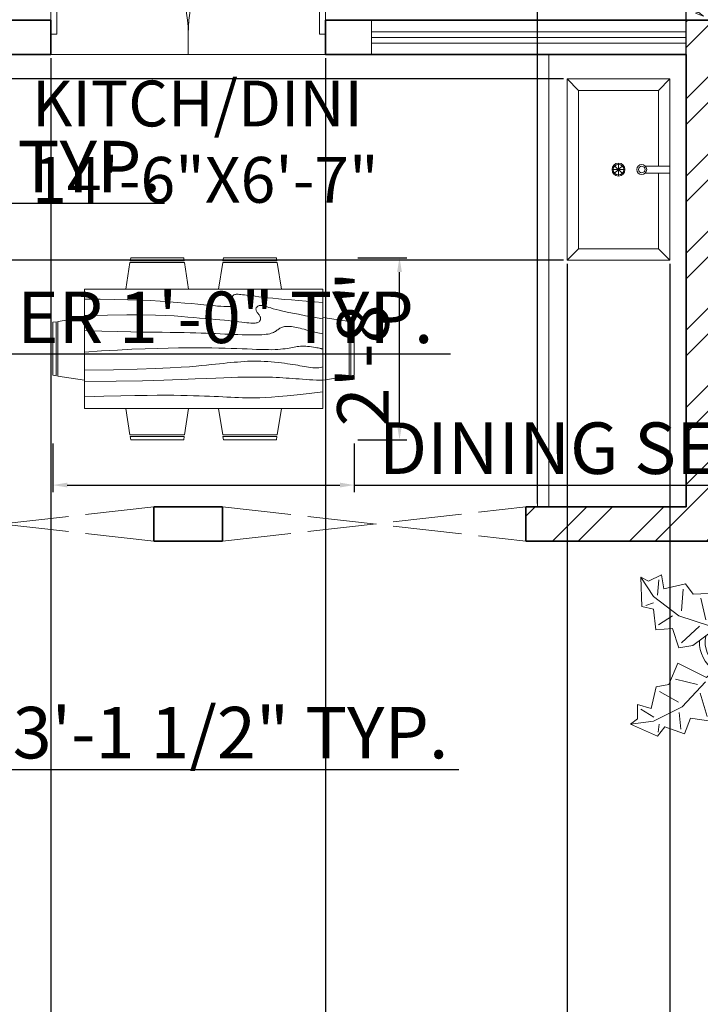
# Model space of a CAD drawing. Units: inches. Extents: x 744 to 1448, y 5126 to 6077.
# Tile 7 of 10: x 1033 to 1152, y 5585 to 5757. Entities that reach past the tile are written whole.
import ezdxf

# ---------------------------------------------------------------- set-up
doc = ezdxf.new("R2010")
doc.units = ezdxf.units.IN
doc.linetypes.add('ACAD_ISO02W100', pattern=[15, 12, -3])
for name, color, linetype, lineweight in [('A-ANNO-DIMS', 2, 'Continuous', 18), ('A-AREA-IDEN', 7, 'Continuous', 18), ('A-DOOR', 4, 'Continuous', 18), ('A-FLOR-CASE', 8, 'Continuous', 18), ('A-FLOR-FIXT', 9, 'Continuous', 18), ('A-FURN', 8, 'Continuous', 18), ('A-WALL', 7, 'Continuous', 35), ('A-WALL-PATT', 252, 'Continuous', 13), ('L-PLNT', 3, 'Continuous', 13)]:
    doc.layers.add(name, color=color, linetype=linetype, lineweight=lineweight)
doc.layers.add('A-GLAZ', color=244, linetype='Continuous', lineweight=18, true_color=0x991b1e)
doc.layers.add('A-WALL-OVHD', color=244, linetype='ACAD_ISO02W100', lineweight=13, true_color=0x991b1e)
doc.styles.get("Standard").update_dxf_attribs({"font": 'arial.ttf'})
doc.dimstyles.new('ISO-25', dxfattribs={"dimtxt": 9, "dimasz": 2.5, "dimexe": 1.25, "dimexo": 0.625, "dimtad": 1, "dimlunit": 3, "dimtxsty": 'Standard', "dimcen": 2.5, "dimadec": 0, "dimazin": 0, "dimtfac": 1, "dimtmove": 0, "dimatfit": 3, "dimfxl": 1, "dimarcsym": 0})

# ---------------------------------------------------------------- blocks, each defined once
blk = doc.blocks.new('*U2')
for p, q in [((0, 0), (0, -6)), ((40, 0), (40, -6))]:
    blk.add_line(p, q)
blk.add_lwpolyline([(0, 0), (0, 40), (1.75, 40), (1.75, 0)], close=True)
blk.add_arc((0, 0), 40, 0, 90)
blk = doc.blocks.new('*U6')
for p, q in [((0, 0), (0, -6)), ((-40, 0), (-40, -6))]:
    blk.add_line(p, q)
blk.add_lwpolyline([(0, 0), (0, 40), (-1.75, 40), (-1.75, 0)], close=True)
blk.add_arc((0, 0), 40, 90, 180)
blk = doc.blocks.new('Dining Set - 36 x 72 in.')
for p, q in [((-22, 27.5), (-22.1562, 26.50042)), ((-22, 27.5), (-6, 27.5)), ((-5.8437, 26.49966), (-6, 27.5)), ((6, 27.5), (5.8438, 26.50042)), ((6, 27.5), (22, 27.5)), ((22.1563, 26.49966), (22, 27.5)), ((-22.2343, 26.00059), (-23.4847, 17.99762)), ((-22.2304, 26), (-5.7608, 26)), ((-5.8416, 26.5), (-22.1534, 26.5)), ((-4.5152, 17.99762), (-5.7655, 25.99926)), ((5.7657, 26.00059), (4.5153, 17.99762)), ((5.7696, 26), (22.2392, 26)), ((22.1584, 26.5), (5.8466, 26.5)), ((23.4848, 17.99762), (22.2345, 25.99926)), ((36, 18), (-36, 18)), ((-36, 18), (-36, -18)), ((36, -18), (36, 18)), ((-44.0006, 8.23428), (-35.9976, 9.48474)), ((44.0006, 8.23428), (35.9976, 9.48474)), ((-45.5, 8), (-44.5004, 8.15617)), ((-45.5, 8), (-45.5, -8)), ((-44.5, -8.15843), (-44.5, 8.15338)), ((-44, 8.23041), (-44, -8.23915)), ((44, 8.23041), (44, -8.23915)), ((44.5, -8.15843), (44.5, 8.15338)), ((45.5, 8), (44.5005, 8.15617)), ((45.5, 8), (45.5, -8)), ((-44.4997, -8.15631), (-45.5, -8)), ((-35.9976, -9.48476), (-43.9993, -8.2345)), ((35.9976, -9.48476), (43.9993, -8.2345)), ((44.4997, -8.15631), (45.5, -8)), ((-36, -18), (36, -18)), ((-22.2343, -26.0006), (-23.4847, -17.99762)), ((-4.5152, -17.99762), (-5.7655, -25.99928)), ((5.7657, -26.0006), (4.5153, -17.99762)), ((23.4848, -17.99762), (22.2345, -25.99928)), ((-22.2304, -26), (-5.7608, -26)), ((-22, -27.5), (-22.1562, -26.50044)), ((-5.8416, -26.5), (-22.1534, -26.5)), ((-5.8437, -26.49967), (-6, -27.5)), ((5.7696, -26), (22.2392, -26)), ((6, -27.5), (5.8438, -26.50044)), ((22.1584, -26.5), (5.8466, -26.5)), ((22.1563, -26.49967), (22, -27.5)), ((-22, -27.5), (-6, -27.5)), ((6, -27.5), (22, -27.5))]:
    blk.add_line(p, q)
for points in [[(-36, 15), (-31.1772, 14.97754), (-26.8079, 14.91406), (-22.8538, 14.81543), (-19.276, 14.6875), (-16.0362, 14.53613), (-13.0957, 14.36718), (-10.4159, 14.18652), (-7.9583, 14), (-5.6904, 13.81315), (-3.6035, 13.63021), (-1.6954, 13.45508), (0.0365, 13.29166), (1.5945, 13.14388), (2.9811, 13.01562), (4.1988, 12.9108), (5.25, 12.83333), (6.1393, 12.78613), (6.8802, 12.76823), (7.4883, 12.77767), (7.9792, 12.8125), (8.3685, 12.87077), (8.6719, 12.95052), (8.9049, 13.0498), (9.0833, 13.16666), (9.2205, 13.29899), (9.3216, 13.44401), (9.3895, 13.59879), (9.4271, 13.76041), (9.4373, 13.92594), (9.4232, 14.09245), (9.3875, 14.257), (9.3333, 14.41666), (9.2638, 14.56917), (9.1836, 14.71484), (9.0975, 14.85465), (9.0104, 14.98958), (8.9272, 15.1206), (8.8529, 15.2487), (8.7922, 15.37483), (8.75, 15.5), (8.7305, 15.62467), (8.7344, 15.74739), (8.7617, 15.86621), (8.8125, 15.97916), (8.8867, 16.08431), (8.9844, 16.17968), (9.1055, 16.26334), (9.25, 16.33333), (9.4189, 16.38802), (9.6172, 16.42708), (9.8506, 16.45052), (10.125, 16.45833), (10.4463, 16.45052), (10.8203, 16.42708), (11.2529, 16.38802), (11.75, 16.33333), (12.3184, 16.26318), (12.9694, 16.17838), (13.7151, 16.07991), (14.5677, 15.96875), (15.5395, 15.84586), (16.6426, 15.71224), (17.8893, 15.56884), (19.2917, 15.41666), (20.859, 15.25667), (22.5879, 15.08984), (24.4721, 14.91715), (26.5052, 14.73958), (28.6809, 14.5581), (30.9929, 14.3737), (33.4347, 14.18733), (36, 14)], [(-36, 10), (-28.9766, 10.14274), (-23.1725, 10.20442), (-18.4241, 10.19775), (-14.5677, 10.13541), (-11.4399, 10.03011), (-8.877, 9.89453), (-6.7154, 9.74137), (-4.7917, 9.58333), (-2.9698, 9.43082), (-1.2246, 9.28515), (0.4415, 9.14534), (2.026, 9.01041), (3.5266, 8.87939), (4.9408, 8.7513), (6.266, 8.62516), (7.5, 8.5), (8.6411, 8.37549), (9.6914, 8.2539), (10.6538, 8.13818), (11.5312, 8.03125), (12.3267, 7.93603), (13.043, 7.85547), (13.6831, 7.79248), (14.25, 7.75), (14.7471, 7.7303), (15.1797, 7.73307), (15.5537, 7.75732), (15.875, 7.80208), (16.1494, 7.86637), (16.3828, 7.94922), (16.5811, 8.04964), (16.75, 8.16666), (16.8944, 8.29915), (17.0143, 8.44531), (17.1089, 8.60319), (17.1771, 8.77083), (17.218, 8.94629), (17.2305, 9.1276), (17.2137, 9.31282), (17.1667, 9.5), (17.0895, 9.6875), (16.987, 9.875), (16.8649, 10.0625), (16.7292, 10.25), (16.5856, 10.4375), (16.4401, 10.625), (16.2985, 10.8125), (16.1667, 11), (16.05, 11.18733), (15.9518, 11.3737), (15.8752, 11.5581), (15.8229, 11.73958), (15.798, 11.91715), (15.8034, 12.08984), (15.842, 12.25667), (15.9167, 12.41666), (16.0295, 12.56836), (16.1784, 12.70833), (16.3605, 12.83268), (16.5729, 12.9375), (16.8127, 13.01888), (17.0768, 13.07291), (17.3625, 13.0957), (17.6667, 13.08333), (17.9894, 13.03312), (18.3418, 12.94726), (18.7382, 12.82918), (19.1927, 12.68229), (19.7195, 12.51001), (20.3327, 12.31575), (21.0465, 12.10294), (21.875, 11.875), (22.8357, 11.63354), (23.959, 11.37304), (25.2786, 11.08618), (26.8282, 10.76562), (28.6414, 10.40405), (30.752, 9.99414), (33.1936, 9.52856), (36, 9)], [(-36, 5.5), (-30.7157, 5.3348), (-26.069, 5.20963), (-21.9946, 5.11767), (-18.4271, 5.05208), (-15.3009, 5.00602), (-12.5508, 4.97265), (-10.1112, 4.94515), (-7.9167, 4.91666), (-5.909, 4.88167), (-4.0586, 4.83984), (-2.3429, 4.79215), (-0.7396, 4.73958), (0.7739, 4.6831), (2.22, 4.6237), (3.6213, 4.56233), (5, 4.5), (6.373, 4.43782), (7.7344, 4.3776), (9.0723, 4.32129), (10.375, 4.27083), (11.6309, 4.22819), (12.8281, 4.19531), (13.9551, 4.17415), (15, 4.16666), (15.954, 4.17448), (16.819, 4.19791), (17.6001, 4.23698), (18.3021, 4.29166), (18.9299, 4.36198), (19.4883, 4.44791), (19.9823, 4.54948), (20.4167, 4.66666), (20.7969, 4.79899), (21.1302, 4.94401), (21.4245, 5.09879), (21.6875, 5.26041), (21.9271, 5.42594), (22.1511, 5.59245), (22.3672, 5.757), (22.5834, 5.91666), (22.8065, 6.06868), (23.0404, 6.21093), (23.2879, 6.34147), (23.5521, 6.45833), (23.8358, 6.55957), (24.142, 6.64323), (24.4735, 6.70735), (24.8334, 6.75), (25.2235, 6.76969), (25.642, 6.76692), (26.0858, 6.74267), (26.5521, 6.69791), (27.0379, 6.63362), (27.5404, 6.55078), (28.0565, 6.45036), (28.5834, 6.33333), (29.1242, 6.19987), (29.7071, 6.04687), (30.3661, 5.87044), (31.1354, 5.66666), (32.0493, 5.43164), (33.142, 5.16146), (34.4475, 4.85221), (36, 4.5)], [(-36, -1), (-30.7915, -0.6591), (-26.0195, -0.38216), (-21.6519, -0.16284), (-17.6563, 0.00521), (-14.0005, 0.12833), (-10.6523, 0.21289), (-7.5796, 0.26522), (-4.75, 0.29166), (-2.134, 0.29793), (0.2878, 0.28711), (2.5317, 0.26163), (4.6146, 0.22396), (6.5529, 0.17651), (8.3633, 0.12174), (10.0623, 0.06209), (11.6667, 0), (13.1899, -0.06201), (14.6341, -0.1211), (15.9982, -0.17432), (17.2813, -0.21875), (18.4823, -0.25147), (19.6003, -0.26953), (20.6343, -0.27002), (21.5834, -0.25), (22.4481, -0.20768), (23.2357, -0.14584), (23.9549, -0.06836), (24.6146, 0.02083), (25.2235, 0.11784), (25.7904, 0.21875), (26.3241, 0.31966), (26.8334, 0.41666), (27.3265, 0.50618), (27.8099, 0.58593), (28.2894, 0.65397), (28.7709, 0.70833), (29.2601, 0.74707), (29.763, 0.76823), (30.2855, 0.76985), (30.8334, 0.75), (31.4088, 0.70784), (31.9994, 0.64713), (32.589, 0.57275), (33.1615, 0.48958), (33.7008, 0.4025), (34.1908, 0.3164), (34.6153, 0.23616), (34.9584, 0.16666), (35.2099, 0.11165), (35.3848, 0.07031), (35.504, 0.04069), (35.5886, 0.02083), (35.6594, 0.00879), (35.7377, 0.0026), (35.8442, 0.00032), (36, 0)], [(-36, -6.5), (-27.1843, -6.31267), (-20.084, -6.1263), (-14.469, -5.9419), (-10.1094, -5.76042), (-6.7752, -5.58285), (-4.2363, -5.41016), (-2.2629, -5.24333), (-0.625, -5.08334), (0.8708, -4.93099), (2.2715, -4.78646), (3.5872, -4.64974), (4.8281, -4.52084), (6.0046, -4.39974), (7.127, -4.28646), (8.2053, -4.18099), (9.25, -4.08334), (10.2705, -3.99382), (11.2734, -3.91407), (12.2647, -3.84603), (13.25, -3.79167), (14.2354, -3.75293), (15.2266, -3.73177), (16.2295, -3.73015), (17.25, -3.75), (18.2912, -3.79248), (19.3451, -3.85547), (20.4009, -3.93604), (21.4479, -4.03125), (22.4754, -4.13819), (23.4727, -4.25391), (24.4289, -4.37549), (25.3334, -4.5), (26.1785, -4.62492), (26.9694, -4.74935), (27.7145, -4.87281), (28.4219, -4.99479), (29.1, -5.11483), (29.7572, -5.23242), (30.4016, -5.34709), (31.0417, -5.45834), (31.6837, -5.56437), (32.3262, -5.65821), (32.9658, -5.73153), (33.599, -5.77604), (34.2224, -5.78345), (34.8327, -5.74545), (35.4264, -5.65373), (36, -5.5)], [(-36, -10), (-26.4022, -9.81299), (-18.4675, -9.62891), (-11.9839, -9.45069), (-6.7396, -9.28125), (-2.5226, -9.12354), (0.8789, -8.98047), (3.6769, -8.85498), (6.0833, -8.75), (8.2767, -8.66765), (10.3021, -8.60677), (12.1712, -8.56543), (13.8958, -8.54167), (15.4876, -8.53353), (16.9583, -8.53907), (18.3197, -8.55632), (19.5834, -8.58334), (20.7616, -8.61841), (21.8685, -8.66081), (22.9188, -8.71004), (23.9271, -8.76563), (24.9081, -8.82707), (25.8763, -8.89388), (26.8465, -8.96558), (27.8334, -9.04167), (28.8474, -9.12118), (29.8828, -9.20117), (30.93, -9.27824), (31.9792, -9.34896), (33.0205, -9.40991), (34.0443, -9.45768), (35.0407, -9.48885), (36, -9.5)], [(-36, -14.5), (-30.0881, -14.33513), (-25.0332, -14.21224), (-20.7312, -14.12647), (-17.0781, -14.07292), (-13.97, -14.04671), (-11.3027, -14.04297), (-8.9724, -14.05681), (-6.875, -14.08334), (-4.9224, -14.11833), (-3.0905, -14.16016), (-1.3709, -14.20785), (0.2448, -14.26042), (1.7647, -14.3169), (3.1973, -14.3763), (4.5507, -14.43767), (5.8333, -14.5), (7.0554, -14.5621), (8.235, -14.62175), (9.3922, -14.67652), (10.5469, -14.72396), (11.7192, -14.76164), (12.929, -14.78711), (14.1965, -14.79794), (15.5417, -14.79167), (16.9933, -14.76424), (18.6152, -14.70508), (20.4804, -14.60197), (22.6615, -14.44271), (25.2312, -14.21509), (28.2624, -13.9069), (31.8277, -13.50594), (36, -13)]]:
    blk.add_lwpolyline(points)
blk = doc.blocks.new('Plant - Rubber or Philodendron')
for p, q in [((13.3837, 12.301), (14.68, 13.9039)), ((14.68, 13.9039), (19.3848, 11.8146)), ((8.8871, 10.7908), (9.9809, 13.4933)), ((9.9809, 13.4933), (13.3837, 12.301)), ((10.5828, 12.6946), (10.8893, 9.7953)), ((14.5816, 13.2037), (14.3848, 11.8033)), ((-16.2005, 11.4774), (-13.9899, 8.1064)), ((-16.2005, 11.4774), (-14.8639, 10.7964)), ((-16.0159, 6.3329), (-16.2005, 11.4774)), ((-14.8639, 10.7964), (-12.6195, 11.8975)), ((-13.3174, 8.325), (-13.0735, 11.0065)), ((-12.6195, 11.8975), (-12.1909, 9.4345)), ((4.6914, 8.8812), (5.3859, 11.2828)), ((5.3859, 11.2828), (8.8871, 10.7908)), ((5.9878, 10.4842), (7.1971, 6.3869)), ((15.3859, 11.3055), (10.3916, 8.7942)), ((15.2875, 10.6053), (17.5907, 9.2105)), ((19.3848, 11.8146), (15.3859, 11.3055)), ((19.3848, 11.8146), (18.1868, 10.9119)), ((18.1868, 10.9119), (18.1925, 8.4119)), ((-12.1909, 9.4345), (-8.3829, 10.3)), ((-8.8369, 9.409), (-9.0894, 5.6095)), ((-8.3829, 10.3), (-7.0549, 8.501)), ((-7.0549, 8.501), (-3.0284, 8.6941)), ((-3.0284, 8.6941), (-3.0709, 3.1041)), ((4.6914, 8.8812), (5.5014, 4.4831)), ((10.3916, 8.7942), (6.2847, 4.4028)), ((15.7909, 9.1065), (14.8995, 5.3044)), ((18.1925, 8.4119), (15.7909, 9.1065)), ((-15.3434, 6.5514), (-13.9984, 6.9884)), ((-13.9899, 8.1064), (-9.5434, 4.7185)), ((-4.8529, 4.012), (-5.7184, 7.82)), ((14.2977, 6.1031), (10.9934, 7.9956)), ((-14.0069, 5.8704), (-16.0159, 6.3329)), ((-13.5868, 2.2894), (-14.0069, 5.8704)), ((14.8995, 5.3044), (12.7005, 4.8994)), ((-13.1329, 3.1804), (-10.6614, 4.727)), ((-9.5434, 4.7185), (-4.1917, 2.9888)), ((2.1141, 0.2298), (5.4346, 3.9146)), ((6.1032, 3.6844), (2.8262, -0.031)), ((5.4346, 3.9146), (5.5014, 4.4831)), ((11.1089, 1.1958), (6.1032, 3.6844)), ((7.7005, 4.8881), (11.5025, 3.9967)), ((12.7005, 4.8994), (11.1089, 1.1958)), ((-10.6784, 2.491), (-13.5868, 2.2894)), ((-9.5858, -0.8715), (-10.6784, 2.491)), ((-9.1318, 0.0195), (-5.9793, 2.9025)), ((-7.1228, -0.443), (-3.5248, 2.2131)), ((-3.5248, 2.2131), (-3.3011, 2.4355)), ((-3.3011, 2.4355), (-0.5306, 1.7947)), ((-3.0709, 3.1041), (0.0797, 2.3163)), ((-0.5306, 1.7947), (-0.2255, -0.5527)), ((-0.5306, 1.7947), (-0.5306, 1.7947)), ((0.0797, 2.3163), (0.4866, -0.031)), ((0.4866, -0.031), (2.1141, 0.2298)), ((-7.1228, -0.443), (-9.5858, -0.8715)), ((-2.019, -3.6148), (-0.2255, -0.5527)), ((-0.9375, -3.1608), (0.5883, -0.8135)), ((0.5883, -0.8135), (2.2447, -2.0916)), ((2.8262, -0.031), (1.3003, -0.5527)), ((1.3003, -0.5527), (2.4193, -1.4655)), ((2.4193, -1.4655), (6.895, -2.1175)), ((11.6605, -0.5413), (6.895, -2.1175)), ((11.6605, -0.5413), (14.1354, -0.8948)), ((14.1354, -0.8948), (14.1354, -4.4304)), ((-4.0579, -6.2781), (-0.9375, -3.1608)), ((2.2447, -2.0916), (6.7108, -2.6626)), ((4.943, -7.9659), (6.7108, -2.6626)), ((12.3677, -6.1981), (7.219, -2.6772)), ((8.3544, -2.7453), (13.1973, -2.1704)), ((-11.3237, -7.2629), (-9.7321, -3.5593)), ((-9.7321, -3.5593), (-4.7264, -6.0479)), ((-2.019, -3.6148), (-4.7264, -6.0479)), ((8.125, -4.0768), (7.7715, -7.9659)), ((14.1354, -4.4304), (16.9638, -5.1375)), ((16.9638, -5.1375), (16.2567, -8.673)), ((-6.3237, -7.2516), (-10.1257, -6.3602)), ((-9.0148, -11.1577), (-4.9047, -6.8122)), ((-4.1246, -6.8466), (-4.0579, -6.2781)), ((-3.3146, -11.2447), (-4.1246, -6.8466)), ((15.5496, -10.7943), (12.3677, -6.1981)), ((16.2567, -5.8446), (13.4283, -6.5517)), ((-14.4141, -11.4699), (-13.5228, -7.6679)), ((-13.5228, -7.6679), (-11.3237, -7.2629)), ((-12.921, -8.4665), (-9.6166, -10.359)), ((8.8321, -9.0266), (4.943, -7.9659)), ((10.2463, -10.4408), (11.6605, -6.9053)), ((-4.611, -12.8477), (-5.8203, -8.7504)), ((9.5392, -11.1479), (8.8321, -9.0266)), ((17.3174, -9.7337), (15.9032, -9.7337)), ((16.2567, -8.673), (18.0245, -9.7337)), ((18.0245, -9.7337), (16.6103, -14.6834)), ((-16.8157, -10.7754), (-14.4141, -11.4699)), ((-16.8101, -13.2754), (-16.8157, -10.7754)), ((-13.9107, -12.9688), (-16.2139, -11.574)), ((-14.0091, -13.669), (-9.0148, -11.1577)), ((-3.3146, -11.2447), (-4.0092, -13.6463)), ((13.4283, -11.5015), (9.5392, -11.1479)), ((13.0748, -13.9763), (13.4283, -11.5015)), ((14.8425, -10.7943), (13.7819, -13.2692)), ((16.6103, -14.6834), (15.5496, -10.7943)), ((-18.008, -14.1781), (-16.8101, -13.2754)), ((-18.008, -14.1781), (-14.0091, -13.669)), ((-9.206, -15.0581), (-9.5126, -12.1588)), ((-7.5103, -13.1543), (-8.6042, -15.8568)), ((-4.0092, -13.6463), (-7.5103, -13.1543)), ((15.5496, -13.6228), (13.0748, -13.9763)), ((16.6103, -14.6834), (15.5496, -13.6228)), ((-13.3032, -16.2674), (-18.008, -14.1781)), ((-12.0069, -14.6645), (-13.3032, -16.2674)), ((-13.2048, -15.5672), (-13.008, -14.1668)), ((-8.6042, -15.8568), (-12.0069, -14.6645))]:
    blk.add_line(p, q)
for centre, radius, start, end in [((0, 0), 6.1275, 34.37569, 120.1028), ((-0.0601, -0.2075), 5.2461, 33.82192, 124.9414), ((-0.2664, 0.1682), 5.2775, 338.4094, 20.03007), ((-0.098, 0.1364), 6.1288, 341.2017, 26.09184), ((0.0308, 0.1664), 6, 178.6147, 235.1169), ((0.0308, 0.1664), 5, 168.1647, 238.6725), ((-0.0234, 0.3825), 6.1492, 242.5812, 331.2714), ((-0.1102, 0.4886), 5.2883, 247.3711, 327.472)]:
    blk.add_arc(centre, radius, start, end)
blk = doc.blocks.new('*U11')
for points in [[(1.24, 12), (0.56, 11.31), (0.76, 10.01), (2.52, 11.05)], [(-4.43, 11.05), (-5.18, 10.36), (-3.96, 9.49), (-2.07, 10.36)], [(-2, 11.66), (-1.6, 10.62), (-0.52, 10.1), (-0.18, 10.62), (-0.79, 10.96)], [(4.14, 11.14), (3.6, 10.01), (4, 9.23), (5.22, 8.71), (6.3, 9.41), (5.08, 10.19), (4.61, 10.01)], [(-5.78, 9.75), (-7.54, 9.23), (-8.01, 7.5), (-6.26, 8.45)], [(-4.84, 8.63), (-3.83, 7.85), (-4.03, 8.97)], [(-1.94, 9.49), (-2.48, 8.97), (-2.27, 8.54), (-1.8, 9.06)], [(0.02, 9.06), (-1.33, 8.54), (-1.73, 7.16), (0.29, 7.76)], [(1.37, 8.54), (3.13, 8.8), (3.8, 7.85), (1.91, 7.76)], [(2.59, 9.93), (1.84, 9.75), (1.64, 9.23), (2.32, 9.41)], [(7.45, 9.32), (7.11, 7.94), (8.52, 7.94)], [(-2.88, 7.5), (-3.15, 6.64), (-2.27, 6.72)], [(1.71, 6.29), (1.71, 7.07), (2.65, 7.5), (2.11, 6.9)], [(4.61, 8.28), (4.54, 7.76), (4.95, 7.59), (4.95, 8.28)], [(6.43, 7.94), (5.49, 7.68), (5.56, 6.21), (6.5, 6.64)], [(-8.14, 6.03), (-9.36, 5.95), (-9.02, 4.73)], [(-5.78, 6.81), (-6.66, 6.21), (-6.52, 5.69)], [(-4.57, 6.38), (-5.45, 4.47), (-3.89, 4.82)], [(0.76, 7.16), (0.09, 6.46), (1.1, 5.95)], [(2.52, 6.81), (2.52, 5.86), (4.41, 5.17), (4.61, 6.72)], [(7.85, 6.81), (7.18, 6.21), (9, 5.51), (9.33, 6.38)], [(4.41, 4.56), (4.27, 3.7), (5.49, 3.26)], [(5.49, 5.51), (5.42, 4.82), (6.16, 5.08)], [(8.12, 4.99), (7.11, 4.65), (6.5, 4.13), (7.38, 3.09), (8.12, 3.52), (7.65, 3.87)], [(8.73, 4.73), (8.19, 4.56), (8.39, 3.87), (8.59, 4.04)], [(10.28, 5.17), (9.2, 4.04), (9, 2.31), (10.48, 0.49), (11.76, 0.41), (10.35, 2.48), (9.33, 2.4), (10.28, 2.83)], [(-11.32, 1.79), (-9.83, 2.31), (-9.63, 3.44), (-10.44, 3.52)], [(-8.21, 3.09), (-8.48, 2.31), (-7.87, 2.57)], [(3.53, 1.88), (2.86, 3.52), (3.8, 3.52)], [(-7, 1.79), (-7.94, 1.53), (-7.47, 0.49)], [(4.27, 2.74), (5.29, 2.66), (4.41, 1.27)], [(5.83, 1.53), (5.02, 0.41), (5.49, -0.02), (6.5, 0.41)], [(7.51, 1.71), (6.91, 1.27), (6.23, 2.14)], [(8.19, 2.57), (7.92, 2.05), (8.66, 1.53)], [(-8.21, 0.41), (-9.43, 0.32), (-9.83, 0.84)], [(8.12, 0.75), (7.51, 0.15), (8.93, -0.28), (9.13, 0.49)], [(7.78, -0.8), (6.43, -1.5), (6.43, -0.72)], [(10.08, -0.63), (9.74, -1.32), (10.48, -0.89)], [(-10.03, -2.71), (-10.64, -3.31), (-10.44, -4.44), (-9.9, -3.49)], [(8.32, -1.75), (7.98, -2.53), (7.58, -2.1)], [(9.33, -1.75), (9.54, -3.74), (10.14, -2.53)], [(-8.28, -5.73), (-6.79, -5.3), (-7, -6.51)], [(9.33, -5.13), (8.46, -6.25), (7.98, -5.22)], [(6.1, -8.94), (6.16, -7.21), (6.91, -6.69), (7.24, -7.38)], [(8.05, -8.07), (8.59, -7.12), (7.92, -7.55)], [(-2.34, -9.2), (-1.26, -8.5), (-0.99, -9.54)], [(5.29, -7.98), (4.61, -8.16), (5.02, -8.94)], [(-4.84, -8.85), (-4.43, -9.45), (-5.99, -9.8)], [(-2.54, -10.06), (-3.02, -10.23), (-1.8, -10.67)], [(4.07, -9.45), (3.53, -9.97), (4.07, -10.58), (4.61, -9.89)], [(6.03, -9.45), (5.42, -9.97), (6.16, -10.15)], [(0.22, -10.58), (0.83, -11.27), (2.59, -11.36)]]:
    blk.add_lwpolyline(points, close=True)
blk = doc.blocks.new('WINDOW-GLASS-55IN')
for p, q in [((0, 2), (55, 2)), ((0, 1), (55, 1)), ((0, 0), (55, 0))]:
    blk.add_line(p, q)
blk = doc.blocks.new('*D35')
at = {"layer": 'A-ANNO-DIMS', "color": 0, "lineweight": -2, "transparency": 16777216}
for p, q in [((949.42, 5630.92), (949.42, 5624.68)), ((986.81, 5630.92), (986.81, 5624.68)), ((951.92, 5625.93), (984.31, 5625.93)), ((986.81, 5625.93), (1109.97, 5625.93))]:
    blk.add_line(p, q, dxfattribs=at)
at = {"layer": 'A-ANNO-DIMS', "color": 0, "transparency": 16777216}
for points in [[(951.92, 5626.35), (951.92, 5625.52), (949.42, 5625.93)], [(984.31, 5626.35), (984.31, 5625.52), (986.81, 5625.93)]]:
    blk.add_solid(points, dxfattribs=at)
at = {"layer": 'Defpoints', "color": 0, "transparency": 16777216}
for p in [(949.42, 5631.54), (986.81, 5631.54), (986.81, 5625.93)]:
    blk.add_point(p, dxfattribs=at)
at = {"layer": 'A-ANNO-DIMS', "color": 0, "transparency": 16777216, "insert": (1049.64, 5631.22), "char_height": 9, "attachment_point": 5}
blk.add_mtext('PLANT 3\'-1 1/2" TYP.', dxfattribs=at)
blk = doc.blocks.new('*D47')
at = {"layer": 'A-ANNO-DIMS', "color": 0, "lineweight": -2, "transparency": 16777216}
for p, q in [((1039.05, 5682.9), (1039.05, 5674.38)), ((1091.7, 5682.9), (1091.7, 5674.38)), ((1041.55, 5675.63), (1089.2, 5675.63)), ((1091.7, 5675.63), (1215.34, 5675.63))]:
    blk.add_line(p, q, dxfattribs=at)
at = {"layer": 'A-ANNO-DIMS', "color": 0, "transparency": 16777216}
for points in [[(1041.55, 5676.05), (1041.55, 5675.22), (1039.05, 5675.63)], [(1089.2, 5676.05), (1089.2, 5675.22), (1091.7, 5675.63)]]:
    blk.add_solid(points, dxfattribs=at)
at = {"layer": 'Defpoints', "color": 0, "transparency": 16777216}
for p in [(1039.05, 5683.53), (1091.7, 5683.53), (1091.7, 5675.63)]:
    blk.add_point(p, dxfattribs=at)
at = {"layer": 'A-ANNO-DIMS', "color": 0, "transparency": 16777216, "insert": (1154.77, 5680.91), "char_height": 9, "attachment_point": 5}
blk.add_mtext('DINING SET 4\'-4 1/2"', dxfattribs=at)
blk = doc.blocks.new('*D48')
at = {"layer": 'A-ANNO-DIMS', "color": 0, "lineweight": -2, "transparency": 16777216}
for p, q in [((1092.32, 5715.35), (1100.85, 5715.35)), ((1099.6, 5686.03), (1099.6, 5712.85)), ((1092.32, 5683.53), (1100.85, 5683.53))]:
    blk.add_line(p, q, dxfattribs=at)
at = {"layer": 'A-ANNO-DIMS', "color": 0, "transparency": 16777216}
for points in [[(1099.18, 5712.85), (1100.01, 5712.85), (1099.6, 5715.35)], [(1099.18, 5686.03), (1100.01, 5686.03), (1099.6, 5683.53)]]:
    blk.add_solid(points, dxfattribs=at)
at = {"layer": 'Defpoints', "color": 0, "transparency": 16777216}
for p in [(1091.7, 5715.35), (1099.6, 5715.35), (1091.7, 5683.53)]:
    blk.add_point(p, dxfattribs=at)
at = {"layer": 'A-ANNO-DIMS', "color": 0, "transparency": 16777216, "insert": (1094.38, 5699.44), "char_height": 9, "attachment_point": 5, "rotation": 90}
blk.add_mtext('2\'-8"', dxfattribs=at)
blk = doc.blocks.new('*D49')
at = {"layer": 'A-ANNO-DIMS', "color": 0, "lineweight": -2, "transparency": 16777216}
for p, q in [((981.78, 5699.72), (981.78, 5697.3)), ((984.28, 5698.55), (991.22, 5698.55)), ((993.72, 5699.72), (993.72, 5697.3)), ((993.72, 5698.55), (1108.52, 5698.55))]:
    blk.add_line(p, q, dxfattribs=at)
at = {"layer": 'A-ANNO-DIMS', "color": 0, "transparency": 16777216}
for points in [[(984.28, 5698.97), (984.28, 5698.14), (981.78, 5698.55)], [(991.22, 5698.97), (991.22, 5698.14), (993.72, 5698.55)]]:
    blk.add_solid(points, dxfattribs=at)
at = {"layer": 'Defpoints', "color": 0, "transparency": 16777216}
for p in [(981.78, 5700.35), (993.72, 5700.35), (993.72, 5698.55)]:
    blk.add_point(p, dxfattribs=at)
at = {"layer": 'A-ANNO-DIMS', "color": 0, "transparency": 16777216, "insert": (1052.37, 5703.77), "char_height": 9, "attachment_point": 5}
blk.add_mtext('BURNER 1\'-0" TYP.', dxfattribs=at)
blk = doc.blocks.new('*D52')
at = {"layer": 'A-ANNO-DIMS', "color": 0, "lineweight": -2, "transparency": 16777216}
for p, q in [((995.46, 5725.22), (995.46, 5726.14)), ((997.42, 5725.22), (997.42, 5726.14)), ((992.96, 5724.89), (990.46, 5724.89)), ((995.46, 5724.89), (997.42, 5724.89)), ((999.92, 5724.89), (1058.53, 5724.89))]:
    blk.add_line(p, q, dxfattribs=at)
at = {"layer": 'A-ANNO-DIMS', "color": 0, "transparency": 16777216}
for points in [[(992.96, 5725.3), (992.96, 5724.47), (995.46, 5724.89)], [(999.92, 5725.3), (999.92, 5724.47), (997.42, 5724.89)]]:
    blk.add_solid(points, dxfattribs=at)
at = {"layer": 'Defpoints', "color": 0, "transparency": 16777216}
for p in [(995.46, 5724.59), (997.42, 5724.89), (997.42, 5724.59)]:
    blk.add_point(p, dxfattribs=at)
at = {"layer": 'A-ANNO-DIMS', "color": 0, "transparency": 16777216, "insert": (1030.47, 5730.11), "char_height": 9, "attachment_point": 5}
blk.add_mtext('0\'-2" TYP.', dxfattribs=at)
blk = doc.blocks.new('*D56')
at = {"layer": 'A-ANNO-DIMS', "color": 0, "lineweight": -2, "transparency": 16777216}
for p, q in [((1038.68, 5750.19), (1038.68, 5125.91)), ((1086.68, 5750.19), (1086.68, 5125.91)), ((1041.18, 5127.16), (1084.18, 5127.16))]:
    blk.add_line(p, q, dxfattribs=at)
at = {"layer": 'A-ANNO-DIMS', "color": 0, "transparency": 16777216}
for points in [[(1041.18, 5127.58), (1041.18, 5126.75), (1038.68, 5127.16)], [(1084.18, 5127.58), (1084.18, 5126.75), (1086.68, 5127.16)]]:
    blk.add_solid(points, dxfattribs=at)
at = {"layer": 'Defpoints', "color": 0, "transparency": 16777216}
for p in [(1038.68, 5750.82), (1086.68, 5750.82), (1086.68, 5127.16)]:
    blk.add_point(p, dxfattribs=at)
at = {"layer": 'A-ANNO-DIMS', "color": 0, "transparency": 16777216, "insert": (1062.68, 5132.38), "char_height": 9, "attachment_point": 5}
blk.add_mtext('4\'-0"', dxfattribs=at)
blk = doc.blocks.new('*D57')
at = {"layer": 'A-ANNO-DIMS', "color": 0, "lineweight": -2, "transparency": 16777216}
for p, q in [((1123.68, 5672.44), (1123.68, 6059.61)), ((1149.68, 5672.44), (1149.68, 6059.61)), ((1126.18, 6058.36), (1147.18, 6058.36))]:
    blk.add_line(p, q, dxfattribs=at)
at = {"layer": 'A-ANNO-DIMS', "color": 0, "transparency": 16777216}
for points in [[(1126.18, 6058.78), (1126.18, 6057.95), (1123.68, 6058.36)], [(1147.18, 6058.78), (1147.18, 6057.95), (1149.68, 6058.36)]]:
    blk.add_solid(points, dxfattribs=at)
at = {"layer": 'Defpoints', "color": 0, "transparency": 16777216}
for p in [(1149.68, 6058.36), (1123.68, 5671.82), (1149.68, 5671.82)]:
    blk.add_point(p, dxfattribs=at)
at = {"layer": 'A-ANNO-DIMS', "color": 0, "transparency": 16777216, "insert": (1136.68, 6063.51), "char_height": 9, "attachment_point": 5}
blk.add_mtext('2\'-2"', dxfattribs=at)
blk = doc.blocks.new('*D58')
at = {"layer": 'A-ANNO-DIMS', "color": 0, "lineweight": -2, "transparency": 16777216}
for p, q in [((1128.86, 5714.27), (1128.86, 5125.91)), ((1146.83, 5714.27), (1146.83, 5125.91)), ((1131.36, 5127.16), (1144.33, 5127.16)), ((1146.83, 5127.16), (1173.66, 5127.16))]:
    blk.add_line(p, q, dxfattribs=at)
at = {"layer": 'A-ANNO-DIMS', "color": 0, "transparency": 16777216}
for points in [[(1131.36, 5127.58), (1131.36, 5126.75), (1128.86, 5127.16)], [(1144.33, 5127.58), (1144.33, 5126.75), (1146.83, 5127.16)]]:
    blk.add_solid(points, dxfattribs=at)
at = {"layer": 'Defpoints', "color": 0, "transparency": 16777216}
for p in [(1128.86, 5714.9), (1146.83, 5714.9), (1146.83, 5127.16)]:
    blk.add_point(p, dxfattribs=at)
at = {"layer": 'A-ANNO-DIMS', "color": 0, "transparency": 16777216, "insert": (1161.49, 5132.38), "char_height": 9, "attachment_point": 5}
blk.add_mtext('1\'-6"', dxfattribs=at)
blk = doc.blocks.new('*D59')
at = {"layer": 'A-ANNO-DIMS', "color": 0, "lineweight": -2, "transparency": 16777216}
for p, q in [((762.28, 5746.58), (762.28, 5795.38)), ((1128.24, 5746.58), (761.03, 5746.58)), ((762.28, 5717.4), (762.28, 5744.08)), ((1128.24, 5714.9), (761.03, 5714.9))]:
    blk.add_line(p, q, dxfattribs=at)
at = {"layer": 'A-ANNO-DIMS', "color": 0, "transparency": 16777216}
for points in [[(761.87, 5744.08), (762.7, 5744.08), (762.28, 5746.58)], [(761.87, 5717.4), (762.7, 5717.4), (762.28, 5714.9)]]:
    blk.add_solid(points, dxfattribs=at)
at = {"layer": 'Defpoints', "color": 0, "transparency": 16777216}
for p in [(762.28, 5746.58), (1128.86, 5746.58), (1128.86, 5714.9)]:
    blk.add_point(p, dxfattribs=at)
at = {"layer": 'A-ANNO-DIMS', "color": 0, "transparency": 16777216, "insert": (757.01, 5772.23), "char_height": 9, "attachment_point": 5, "rotation": 90}
blk.add_mtext('2\'-7 1/2"', dxfattribs=at)

msp = doc.modelspace()

# ---------------------------------------------------------------- hatches: boundary and pattern name
at = {"layer": 'A-WALL-PATT'}
h = msp.add_hatch(dxfattribs=at)
h.set_pattern_fill('ANSI32', color=256)
h.paths.add_polyline_path([(813.684, 5750.816), (876.684, 5750.816), (876.684, 5756.816), (813.684, 5756.816), (813.684, 5812.816), (909.684, 5812.816), (909.684, 5795.316), (915.684, 5795.316), (915.684, 5812.816), (1209.684, 5812.816), (1209.684, 5795.316), (1215.684, 5795.316), (1215.684, 5812.816), (1311.684, 5812.816), (1311.684, 5756.816), (1248.684, 5756.816), (1248.684, 5750.816), (1311.684, 5750.816), (1311.684, 5570.816), (1179.044, 5570.816), (1179.044, 5564.816), (1311.684, 5564.816), (1311.684, 5383.316), (1260.684, 5383.316), (1260.684, 5377.316), (1311.684, 5377.316), (1311.684, 5320.316), (1227.684, 5320.316), (1227.684, 5333.816), (1221.684, 5333.816), (1221.684, 5314.316), (1320.684, 5314.316), (1320.684, 5821.816), (804.684, 5821.816), (804.684, 5472.316), (926.184, 5472.316), (926.184, 5481.316), (813.684, 5481.316), (813.684, 5581.616), (946.284, 5581.616), (946.284, 5587.616), (813.684, 5587.616)])
h.paths.add_polyline_path([(1155.684, 5525.816), (1149.684, 5525.816), (1149.684, 5481.316), (1025.184, 5481.316), (1025.184, 5475.316), (1146.684, 5475.316), (1146.684, 5323.316), (1118.788, 5323.316), (1118.788, 5314.316), (1146.684, 5314.316), (1155.684, 5314.316), (1155.684, 5374.316), (1170.35, 5374.316), (1170.35, 5383.316), (1155.684, 5383.316)], flags=17)
h.paths.add_polyline_path([(1230.684, 5383.316), (1213.35, 5383.316), (1213.35, 5374.316), (1221.684, 5374.316), (1221.684, 5363.816), (1226.184, 5363.816), (1227.684, 5363.816), (1227.684, 5377.316), (1230.684, 5377.316)], flags=17)
h.paths.add_polyline_path([(1185.684, 5671.816), (1155.684, 5671.816), (1155.684, 5750.816), (1161.575, 5750.816), (1161.575, 5756.816), (1157.542, 5756.816), (1157.847, 5756.715), (1155.79, 5756.816), (1149.684, 5756.816), (1149.684, 5750.816), (1149.684, 5671.816), (1121.684, 5671.816), (1121.684, 5665.816), (1179.684, 5665.816), (1179.684, 5609.816), (1185.684, 5609.816)], flags=17)
h.paths.add_polyline_path([(1003.684, 5671.816), (975.684, 5671.816), (975.684, 5750.816), (975.684, 5756.816), (965.205, 5756.816), (965.205, 5750.816), (969.684, 5750.816), (969.684, 5671.816), (939.684, 5671.816), (939.684, 5626.616), (945.684, 5626.616), (945.684, 5665.816), (1003.684, 5665.816)], flags=17)
h.paths.add_polyline_path([(915.684, 5774.316), (909.684, 5774.316), (909.684, 5756.816), (906.684, 5756.816), (906.684, 5752.316), (906.684, 5750.816), (922.205, 5750.816), (922.205, 5756.816), (915.684, 5756.816)], flags=17)
h.paths.add_polyline_path([(1215.684, 5774.316), (1209.684, 5774.316), (1209.684, 5756.816), (1204.575, 5756.816), (1204.575, 5750.816), (1218.684, 5750.816), (1218.684, 5756.816), (1215.684, 5756.816)], flags=17)
h.paths.add_polyline_path([(1063.788, 5323.316), (1025.184, 5323.316), (1025.184, 5314.316), (1063.788, 5314.316)])
h.paths.add_polyline_path([(986.184, 5475.316), (989.184, 5475.316), (989.184, 5481.316), (974.184, 5481.316), (974.184, 5475.916), (974.184, 5472.316), (977.184, 5472.316), (977.184, 5314.316), (989.184, 5314.316), (989.184, 5319.716), (989.184, 5323.316), (986.184, 5323.316)])

# ---------------------------------------------------------------- linework, layer by layer
at = {"layer": 'A-DOOR'}
msp.add_line((1038.684, 5750.816), (1086.684, 5750.816), dxfattribs=at)
at = {"layer": 'A-FLOR-CASE'}
for p, q in [((1123.684, 5671.816), (1123.684, 5750.816)), ((1125.684, 5671.816), (1125.684, 5750.816))]:
    msp.add_line(p, q, dxfattribs=at)
at = {"layer": 'A-FLOR-FIXT'}
for p, q in [((1130.864, 5744.584), (1128.864, 5746.584)), ((1144.829, 5744.584), (1146.829, 5746.584)), ((1137.013, 5729.975), (1138.681, 5731.506)), ((1138.673, 5729.966), (1137.021, 5731.514)), ((1137.847, 5731.872), (1137.847, 5729.608)), ((1146.829, 5731.34), (1142.541, 5731.34)), ((1136.715, 5730.74), (1138.979, 5730.74)), ((1146.829, 5730.14), (1142.541, 5730.14)), ((1130.864, 5716.896), (1128.864, 5714.896)), ((1144.829, 5716.896), (1146.829, 5714.896))]:
    msp.add_line(p, q, dxfattribs=at)
msp.add_lwpolyline([(1128.864, 5746.584), (1146.829, 5746.584), (1146.829, 5714.896), (1128.864, 5714.896)], close=True, dxfattribs=at)
msp.add_lwpolyline([(1144.829, 5730.14), (1144.829, 5716.896), (1130.864, 5716.896), (1130.864, 5744.584), (1144.829, 5744.584), (1144.829, 5731.34)], dxfattribs=at)
for centre, radius in [((1137.847, 5730.74), 1.132), ((1137.847, 5730.74), 0.932), ((1141.904, 5730.74), 0.875), ((1141.904, 5730.74), 0.575)]:
    msp.add_circle(centre, radius, dxfattribs=at)
at = {"layer": 'A-GLAZ'}
msp.add_lwpolyline([(1094.684, 5756.816), (1149.684, 5756.816), (1149.684, 5750.816), (1094.684, 5750.816)], close=True, dxfattribs=at)
at = {"layer": 'A-WALL'}
for p, q in [((915.684, 5756.816), (1038.684, 5756.816)), ((1038.684, 5750.816), (1038.684, 5756.816)), ((1086.684, 5750.816), (1086.684, 5756.816)), ((1086.684, 5756.816), (1209.684, 5756.816)), ((975.684, 5750.816), (1038.684, 5750.816)), ((1086.684, 5750.816), (1149.684, 5750.816)), ((1149.684, 5671.816), (1149.684, 5750.816)), ((1056.684, 5665.816), (1056.684, 5671.816)), ((1056.684, 5671.816), (1068.684, 5671.816)), ((1068.684, 5665.816), (1068.684, 5671.816)), ((1121.684, 5665.816), (1121.684, 5671.816)), ((1121.684, 5671.816), (1149.684, 5671.816)), ((1056.684, 5665.816), (1068.684, 5665.816)), ((1121.684, 5665.816), (1179.684, 5665.816))]:
    msp.add_line(p, q, dxfattribs=at)
at = {"layer": 'A-WALL-OVHD'}
for p, q in [((1056.684, 5665.816), (1003.684, 5671.816)), ((1056.684, 5671.816), (1003.684, 5665.816)), ((1068.684, 5671.816), (1121.684, 5665.816)), ((1068.684, 5665.816), (1121.684, 5671.816))]:
    msp.add_line(p, q, dxfattribs=at)

# ---------------------------------------------------------------- block references
at = {"layer": 'A-DOOR', "xscale": 0.6, "yscale": 0.6, "zscale": 0.6}
for name, p in [('*U2', (1038.684, 5754.416)), ('*U6', (1086.684, 5754.416))]:
    msp.add_blockref(name, p, dxfattribs=at)
at = {"layer": 'A-FURN', "xscale": 0.5785943029303497, "yscale": 0.5785943029303497, "zscale": 0.5785943029303497}
msp.add_blockref('Dining Set - 36 x 72 in.', (1065.374, 5699.441), dxfattribs=at)
at = {"layer": 'A-GLAZ', "rotation": 180}
msp.add_blockref('WINDOW-GLASS-55IN', (1149.684, 5754.816), dxfattribs=at)
at = {"layer": 'L-PLNT', "xscale": 1.172842970614158, "yscale": 1.172842970614158, "zscale": 1.172842970614158}
msp.add_blockref('*U11', (1154.815, 5770.036), dxfattribs=at)
at = {"layer": 'L-PLNT'}
msp.add_blockref('Plant - Rubber or Philodendron', (1157.959, 5648.06), dxfattribs=at)

# ---------------------------------------------------------------- texts
at = {"layer": 'A-AREA-IDEN', "insert": (1035.419, 5746.286), "char_height": 8, "attachment_point": 1}
msp.add_mtext_dynamic_manual_height_columns('KITCH/DINI\\P14\'-6"X6\'-7"', width=61.27377, gutter_width=12.5, heights=[0], dxfattribs=at)

# ---------------------------------------------------------------- dimensions: what is measured, and where the dimension line sits
at = {"layer": 'A-ANNO-DIMS'}
for base, p1, p2, picture, middle in [((1149.684, 6058.363), (1123.684, 5671.816), (1149.684, 5671.816), '*D57', (1136.684, 6063.507)), ((1086.684, 5127.162), (1038.684, 5750.816), (1086.684, 5750.816), '*D56', (1062.684, 5132.383)), ((1146.829, 5127.162), (1128.864, 5714.896), (1146.829, 5714.896), '*D58', (1161.493, 5132.383))]:
    dim = msp.add_linear_dim(base=base, p1=p1, p2=p2, dimstyle='ISO-25', override={"dimdec": 1, "dimlfac": 1, "dimrnd": 0, "dimzin": 1, "dimdsep": 46, "dimlunit": 4, "dimfrac": 2}, dxfattribs=at)
    dim.commit()
    dim.dimension.update_dxf_attribs({"geometry": picture, "text_midpoint": middle})
for base, p1, p2, picture, middle in [((762.284, 5746.584), (1128.864, 5714.896), (1128.864, 5746.584), '*D59', (757.006, 5772.234)), ((1099.597, 5715.352), (1091.7, 5683.53), (1091.7, 5715.352), '*D48', (1094.377, 5699.441))]:
    dim = msp.add_linear_dim(base=base, p1=p1, p2=p2, angle=90, dimstyle='ISO-25', override={"dimdec": 1, "dimlfac": 1, "dimrnd": 0, "dimzin": 1, "dimdsep": 46, "dimlunit": 4, "dimfrac": 2}, dxfattribs=at)
    dim.commit()
    dim.dimension.update_dxf_attribs({"geometry": picture, "text_midpoint": middle})
for base, p1, p2, text, picture, middle in [((997.419, 5724.887), (995.462, 5724.594), (997.419, 5724.594), '<> TYP.', '*D52', (1030.474, 5730.108)), ((993.724, 5698.555), (981.782, 5700.346), (993.724, 5700.346), 'BURNER <> TYP.', '*D49', (1052.372, 5703.775)), ((1091.7, 5675.632), (1039.048, 5683.53), (1091.7, 5683.53), 'DINING SET <>', '*D47', (1154.77, 5680.91)), ((986.815, 5625.935), (949.422, 5631.544), (986.815, 5631.544), 'PLANT <> TYP.', '*D35', (1049.64, 5631.216))]:
    dim = msp.add_linear_dim(base=base, p1=p1, p2=p2, text=text, dimstyle='ISO-25', override={"dimdec": 1, "dimlfac": 1, "dimrnd": 0, "dimzin": 1, "dimdsep": 46, "dimlunit": 4, "dimfrac": 2}, dxfattribs=at)
    dim.commit()
    dim.dimension.update_dxf_attribs({"geometry": picture, "text_midpoint": middle})

doc.saveas('drawing.dxf')
